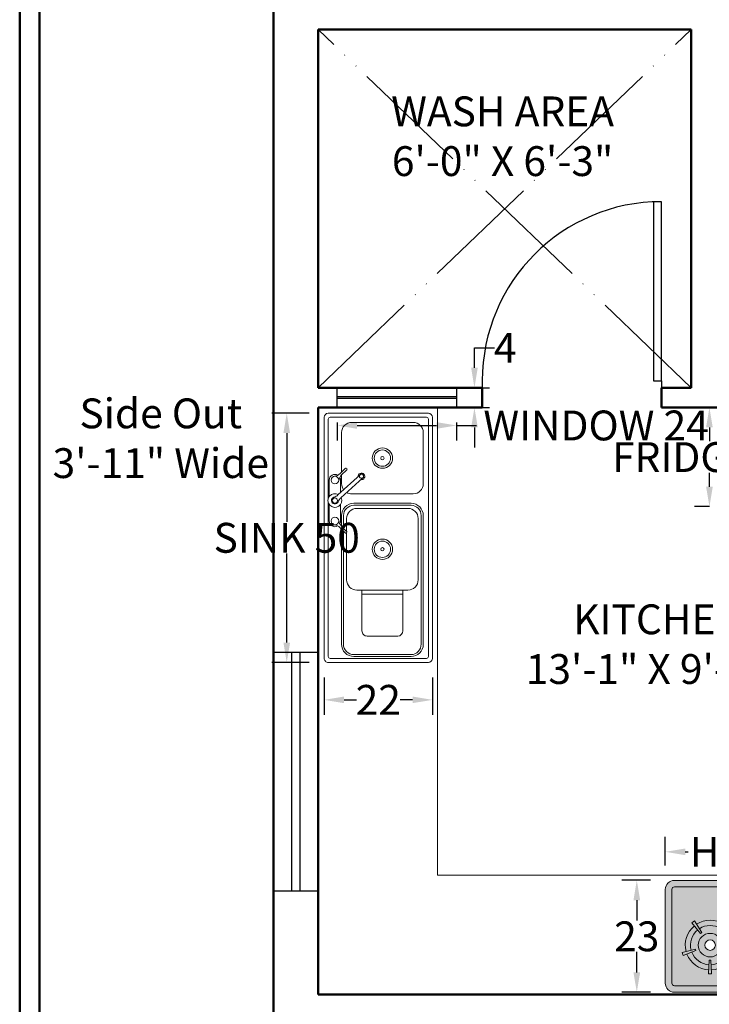
# Model space of a CAD drawing. Units: inches. Extents: x -466983 to 1020, y 324 to 318697.
# Tile 7 of 97: x 392 to 530, y 629 to 827. Entities that reach past the tile are written whole.
import ezdxf

# ---------------------------------------------------------------- set-up
doc = ezdxf.new("R2010")
doc.units = ezdxf.units.IN
doc.header["$MEASUREMENT"] = 0
doc.linetypes.add('ACAD_ISO05W100', pattern=[33, 24, -3, 0, -3, 0, -3])
for name, color, linetype, lineweight in [('A-ANNO-DIMS', 2, 'Continuous', 18), ('A-ANNO-SYMB', 252, 'ACAD_ISO05W100', 18), ('A-AREA-IDEN', 7, 'Continuous', 25), ('A-DOOR', 3, 'Continuous', 25), ('A-EQPM', 8, 'Continuous', 18), ('A-FLOR-FIXT', 9, 'Continuous', 18), ('A-FLOR-PATT', 252, 'Continuous', 13), ('A-GLAZ', 4, 'Continuous', 25), ('A-WALL', 7, 'Continuous', 50)]:
    doc.layers.add(name, color=color, linetype=linetype, lineweight=lineweight)
doc.styles.get("Standard").update_dxf_attribs({"font": 'arial.ttf'})
doc.dimstyles.get("Standard").update_dxf_attribs({"dimtxt": 6, "dimasz": 4, "dimexe": 3, "dimexo": 3, "dimgap": 0.09, "dimtad": 0, "dimtih": 1, "dimtoh": 1, "dimdec": 1, "dimzin": 0, "dimdsep": 46, "dimlunit": 3, "dimtxsty": 'Standard', "dimcen": 0.09, "dimadec": 0, "dimazin": 0, "dimtfac": 1, "dimtdec": 1, "dimtofl": 0, "dimtmove": 0, "dimatfit": 3, "dimfxl": 1, "dimtolj": 1, "dimtzin": 0, "dimarcsym": 0})

# ---------------------------------------------------------------- blocks, each defined once
blk = doc.blocks.new('Window 4 ft')
for p, q in [((1224.69, 893.77), (1233.69, 893.77)), ((1224.69, 845.77), (1224.69, 893.77)), ((1228.39, 845.77), (1228.39, 893.77)), ((1229.99, 893.77), (1229.99, 845.77)), ((1233.69, 893.77), (1233.69, 845.77)), ((1233.69, 845.77), (1224.69, 845.77))]:
    blk.add_line(p, q)
blk = doc.blocks.new('Window 4 inches')
for p, q in [((1548.16, 1036.06), (1572.16, 1036.06)), ((1548.16, 1032.06), (1548.16, 1036.06)), ((1572.16, 1036.06), (1572.16, 1032.06)), ((1548.16, 1034.26), (1572.16, 1034.26)), ((1572.16, 1033.86), (1548.16, 1033.86)), ((1572.16, 1032.06), (1548.16, 1032.06))]:
    blk.add_line(p, q)
blk = doc.blocks.new('*U39')
for p, q in [((0, 0), (0, -6)), ((-40, 0), (-40, -6))]:
    blk.add_line(p, q)
blk.add_lwpolyline([(0, 0), (0, 40), (-1.75, 40), (-1.75, 0)], close=True)
blk.add_arc((0, 0), 40, 90, 180)
blk = doc.blocks.new('Kitchen Sink')
at = {"color": 0}
for p, q in [((2657.86, 1007.76), (2657.86, 1030.74)), ((2714.14, 1031.68), (2658.8, 1031.68)), ((2713.67, 1030.74), (2659.27, 1030.74)), ((2715.08, 1007.76), (2715.08, 1030.74)), ((2658.8, 1030.27), (2658.8, 1008.23)), ((2674.04, 1029.57), (2662.32, 1029.57)), ((2710.89, 1029.57), (2681.35, 1029.57)), ((2710.89, 1029.1), (2681.35, 1029.1)), ((2696.12, 1028.39), (2682.05, 1028.39)), ((2714.14, 1008.23), (2714.14, 1030.27)), ((2659.97, 1027.22), (2659.97, 1013.15)), ((2676.39, 1027.22), (2676.39, 1013.15)), ((2678.54, 1026.75), (2678.54, 1013.62)), ((2679.01, 1026.75), (2679.01, 1013.62)), ((2679.71, 1026.05), (2679.71, 1014.32)), ((2698.47, 1026.05), (2698.47, 1014.32)), ((2713.28, 1013.62), (2713.28, 1026.75)), ((2713.71, 1013.62), (2713.71, 1026.75)), ((2698.47, 1024.88), (2707.85, 1024.88)), ((2699.4, 1024.88), (2699.4, 1015.5)), ((2709.02, 1016.67), (2709.02, 1023.7)), ((2676.63, 1009.99), (2672.02, 1015.05)), ((2677.32, 1010.63), (2672.71, 1015.68)), ((2698.47, 1015.5), (2707.85, 1015.5)), ((2671.4, 1010.81), (2662.32, 1010.81)), ((2671.7, 1010.5), (2670.59, 1011.62)), ((2672.03, 1010.83), (2670.93, 1011.95)), ((2674.04, 1010.81), (2672.05, 1010.81)), ((2673.22, 1010.59), (2676.08, 1010.59)), ((2678.79, 1010.59), (2682.6, 1010.59)), ((2681.35, 1011.24), (2684.25, 1011.24)), ((2681.35, 1010.81), (2683.82, 1010.81)), ((2684.99, 1011.98), (2682.05, 1011.98)), ((2683.81, 1010.81), (2684.94, 1011.91)), ((2684.14, 1010.47), (2685.27, 1011.58)), ((2684.49, 1010.81), (2710.89, 1010.81)), ((2684.92, 1011.24), (2710.89, 1011.24)), ((2696.12, 1011.98), (2685.33, 1011.98)), ((2673.22, 1007.97), (2677.03, 1007.97)), ((2678.79, 1007.97), (2682.6, 1007.97)), ((2658.8, 1006.82), (2714.14, 1006.82)), ((2659.27, 1007.76), (2677.51, 1007.76)), ((2678.32, 1007.76), (2713.67, 1007.76))]:
    blk.add_line(p, q, dxfattribs=at)
for centre, radius in [((2668.18, 1020.19), 2.34), ((2668.18, 1020.19), 1.88), ((2689.09, 1020.19), 2.34), ((2689.09, 1020.19), 1.88), ((2668.18, 1020.19), 0.399), ((2689.09, 1020.19), 0.399), ((2672.33, 1015.4), 0.471), ((2673.22, 1009.28), 0.878), ((2682.6, 1009.28), 0.878), ((2677.91, 1009.28), 0.601)]:
    blk.add_circle(centre, radius, dxfattribs=at)
for centre, radius, start, end in [((2658.8, 1030.74), 0.938, 90, 180), ((2659.27, 1030.27), 0.469, 90, 180), ((2713.67, 1030.27), 0.469, 0, 90), ((2714.14, 1030.74), 0.938, 0, 90), ((2662.32, 1027.22), 2.34, 90, 180), ((2674.04, 1027.22), 2.34, 0, 90), ((2681.35, 1026.75), 2.81, 90, 180), ((2681.35, 1026.75), 2.34, 90, 180), ((2682.05, 1026.05), 2.34, 90, 180), ((2696.12, 1026.05), 2.34, 0, 90), ((2710.89, 1026.75), 2.81, 0, 90), ((2710.87, 1026.68), 2.41, 1.6247, 89.3271), ((2707.85, 1023.7), 1.17, 0, 90), ((2672.37, 1015.37), 0.761, 350.3658, 274.3209), ((2707.85, 1016.67), 1.17, 270, 0), ((2662.32, 1013.15), 2.34, 180, 270), ((2674.04, 1013.15), 2.34, 330.2915, 0), ((2681.35, 1013.62), 2.81, 180, 270), ((2681.42, 1013.65), 2.41, 180.6729, 268.3753), ((2682.05, 1014.32), 2.34, 180, 270), ((2696.12, 1014.32), 2.34, 270, 0), ((2710.89, 1013.62), 2.81, 270, 0), ((2710.89, 1013.62), 2.38, 270, 0), ((2670.71, 1011.84), 0.248, 25.7239, 243.2674), ((2670.03, 1008.85), 2.34, 7.6523, 44.4956), ((2673.71, 1012.47), 2.34, 224.4956, 261.339), ((2673.22, 1009.28), 1.31, 90, 119.8816), ((2674.04, 1013.15), 2.34, 270, 307.0737), ((2677.91, 1009.28), 1.58, 149.6444, 115.0423), ((2679.06, 1012.21), 2.34, 222.3434, 248.6112), ((2682.17, 1012.48), 2.34, 277.6523, 314.4956), ((2682.6, 1009.28), 1.31, 59.1097, 90), ((2685.79, 1008.8), 2.34, 134.4956, 171.339), ((2685.16, 1011.8), 0.248, 295.7239, 153.2674), ((2696.12, 1014.32), 2.34, 270, 271.1456), ((2659.27, 1008.23), 0.469, 180, 270), ((2673.22, 1009.28), 1.31, 149.1097, 270), ((2674.9, 1008.41), 2.34, 16.0755, 42.3434), ((2677.91, 1009.28), 0.793, 196.0755, 68.6112), ((2682.6, 1009.28), 1.31, 270, 29.8816), ((2713.67, 1008.23), 0.469, 270, 0), ((2658.8, 1007.76), 0.938, 180, 270), ((2714.14, 1007.76), 0.938, 270, 0)]:
    blk.add_arc(centre, radius, start, end, dxfattribs=at)
blk = doc.blocks.new('Gas Stove')
h = blk.add_hatch(color=256)
h.dxf.hatch_style = 1
h.paths.add_polyline_path([(13032.81, 10915.17, 0.414214), (13029.34, 10918.64), (12963.86, 10918.64, 0.414214), (12960.39, 10915.17), (12960.39, 10879.45, 0.414214), (12963.86, 10875.98), (13029.34, 10875.98, 0.414214), (13032.81, 10879.45)])
h.paths.add_polyline_path([(13030.33, 10879.45, -0.414214), (13029.34, 10878.46), (12963.86, 10878.46, -0.414214), (12962.87, 10879.45), (12962.87, 10915.17, -0.414214), (12963.86, 10916.16), (13029.34, 10916.16, -0.414214), (13030.33, 10915.17)], flags=16)
h.paths.add_polyline_path([(13026, 10904.63), (13026.36, 10903.5), (13024.89, 10903.11, -0.295473), (13021.71, 10893.34), (13022.68, 10892.15), (13021.71, 10891.45), (13020.89, 10892.74, -0.295473), (13010.61, 10892.74), (13009.78, 10891.45), (13008.82, 10892.15), (13009.79, 10893.34, -0.295473), (13006.61, 10903.11), (13005.13, 10903.5), (13005.5, 10904.63), (13006.93, 10904.08, -0.295473), (13015.24, 10910.12), (13015.15, 10911.64), (13016.34, 10911.64), (13016.26, 10910.12, -0.295473), (13024.57, 10904.08)], flags=0)
h.paths.add_polyline_path([(13020.24, 10900.68, -1), (13011.25, 10900.68, -1)], flags=0)
h.paths.add_polyline_path([(13017.76, 10900.68, -1), (13013.73, 10900.68, -1)], flags=0)
h.paths.add_polyline_path([(13001.07, 10889.32), (13001.07, 10886.1), (12992.13, 10886.1), (12992.13, 10889.32)], flags=0)
h.paths.add_polyline_path([(13001.08, 10880.42), (13001.08, 10880.13), (13000.33, 10880.13), (13000.33, 10880.42, -0.820702), (13000.33, 10884.1), (13000.33, 10884.41), (13001.08, 10884.41), (13001.08, 10884.1, -0.816133)], flags=0)
h.paths.add_polyline_path([(12988.06, 10903.5), (12986.59, 10903.11, -0.295473), (12983.41, 10893.34), (12984.38, 10892.15), (12983.41, 10891.45), (12982.59, 10892.74, -0.295473), (12972.31, 10892.74), (12971.48, 10891.45), (12970.52, 10892.15), (12971.49, 10893.34, -0.295473), (12968.31, 10903.11), (12966.83, 10903.5), (12967.2, 10904.63), (12968.63, 10904.08, -0.295473), (12976.94, 10910.12), (12976.85, 10911.64), (12978.04, 10911.64), (12977.96, 10910.12, -0.295473), (12986.27, 10904.08), (12987.7, 10904.63)], flags=0)
h.paths.add_polyline_path([(12992.89, 10880.42), (12992.89, 10880.13), (12992.14, 10880.13), (12992.14, 10880.42, -0.816133), (12992.14, 10884.1), (12992.14, 10884.41), (12992.89, 10884.41), (12992.89, 10884.1, -0.820702)], flags=0)
h.paths.add_polyline_path([(12981.94, 10900.68, -1), (12972.95, 10900.68, -1)], flags=0)
h.paths.add_polyline_path([(12979.46, 10900.68, -1), (12975.43, 10900.68, -1)], flags=0)
h = blk.add_hatch(color=0)
h.dxf.hatch_style = 1
h.set_gradient(color1=(192, 192, 192), color2=(0, 0, 0))
h.paths.add_polyline_path([(13030.33, 10915.17, 0.414214), (13029.34, 10916.16), (12963.86, 10916.16, 0.414214), (12962.87, 10915.17), (12962.87, 10879.45, 0.414214), (12963.86, 10878.46), (13029.34, 10878.46, 0.414214), (13030.33, 10879.45)])
h.paths.add_polyline_path([(12987.7, 10904.63), (12988.06, 10903.5), (12986.59, 10903.11, -0.295473), (12983.41, 10893.34), (12984.38, 10892.15), (12983.41, 10891.45), (12982.59, 10892.74, -0.295473), (12972.31, 10892.74), (12971.48, 10891.45), (12970.52, 10892.15), (12971.49, 10893.34, -0.295473), (12968.31, 10903.11), (12966.83, 10903.5), (12967.2, 10904.63), (12968.63, 10904.08, -0.295473), (12976.94, 10910.12), (12976.85, 10911.64), (12978.04, 10911.64), (12977.96, 10910.12, -0.295473), (12986.27, 10904.08)], flags=16)
h.paths.add_polyline_path([(13005.5, 10904.63), (13006.93, 10904.08, -0.295473), (13015.24, 10910.12), (13015.15, 10911.64), (13016.34, 10911.64), (13016.26, 10910.12, -0.295473), (13024.57, 10904.08), (13026, 10904.63), (13026.36, 10903.5), (13024.89, 10903.11, -0.295473), (13021.71, 10893.34), (13022.68, 10892.15), (13021.71, 10891.45), (13020.89, 10892.74, -0.295473), (13010.61, 10892.74), (13009.78, 10891.45), (13008.82, 10892.15), (13009.79, 10893.34, -0.295473), (13006.61, 10903.11), (13005.13, 10903.5)], flags=16)
h.paths.add_polyline_path([(12981.94, 10900.68, -1), (12972.95, 10900.68, -1)], flags=0)
h.paths.add_polyline_path([(12979.46, 10900.68, -1), (12975.43, 10900.68, -1)], flags=0)
h.paths.add_polyline_path([(13020.24, 10900.68, -1), (13011.25, 10900.68, -1)], flags=0)
h.paths.add_polyline_path([(13017.76, 10900.68, -1), (13013.73, 10900.68, -1)], flags=0)
h.paths.add_polyline_path([(13001.07, 10889.32), (13001.07, 10886.1), (12992.13, 10886.1), (12992.13, 10889.32)], flags=16)
h.paths.add_polyline_path([(12992.89, 10884.41), (12992.89, 10884.1, -0.820702), (12992.89, 10880.42), (12992.89, 10880.13), (12992.14, 10880.13), (12992.14, 10880.42, -0.816133), (12992.14, 10884.1), (12992.14, 10884.41)], flags=16)
h.paths.add_polyline_path([(13000.33, 10884.41), (13001.08, 10884.41), (13001.08, 10884.1, -0.816133), (13001.08, 10880.42), (13001.08, 10880.13), (13000.33, 10880.13), (13000.33, 10880.42, -0.820702), (13000.33, 10884.1)], flags=16)
h.paths.add_polyline_path([(13022.97, 10902.61), (13021.31, 10902.17), (13021.12, 10902.73), (13022.72, 10903.36, 0.295997), (13016.14, 10908.14), (13016.04, 10906.42), (13015.45, 10906.42), (13015.35, 10908.14, 0.295997), (13008.78, 10903.36), (13010.38, 10902.73), (13010.19, 10902.17), (13008.53, 10902.61, 0.295997), (13011.04, 10894.87), (13012.13, 10896.2), (13012.61, 10895.85), (13011.68, 10894.41, 0.295997), (13019.82, 10894.41), (13018.89, 10895.85), (13019.37, 10896.2), (13020.45, 10894.87, 0.295997)], flags=0)
h = blk.add_hatch(color=256)
h.dxf.hatch_style = 1
h.set_gradient(color1=(237, 238, 153), color2=(128, 128, 128), name='INVSPHERICAL')
h.paths.add_polyline_path([(13030.33, 10915.17, 0.414214), (13029.34, 10916.16), (12963.86, 10916.16, 0.414214), (12962.87, 10915.17), (12962.87, 10879.45, 0.414214), (12963.86, 10878.46), (13029.34, 10878.46, 0.414214), (13030.33, 10879.45)])
h.paths.add_polyline_path([(12986.27, 10904.08), (12987.7, 10904.63), (12988.06, 10903.5), (12986.59, 10903.11, -0.295473), (12983.41, 10893.34), (12984.38, 10892.15), (12983.41, 10891.45), (12982.59, 10892.74, -0.295473), (12972.31, 10892.74), (12971.48, 10891.45), (12970.52, 10892.15), (12971.49, 10893.34, -0.295473), (12968.31, 10903.11), (12966.83, 10903.5), (12967.2, 10904.63), (12968.63, 10904.08, -0.295473), (12976.94, 10910.12), (12976.85, 10911.64), (12978.04, 10911.64), (12977.96, 10910.12, -0.295473)], flags=16)
h.paths.add_polyline_path([(12981.94, 10900.68, -1), (12972.95, 10900.68, -1)], flags=0)
h.paths.add_polyline_path([(12979.46, 10900.68, -1), (12975.43, 10900.68, -1)], flags=0)
h.paths.add_polyline_path([(13005.5, 10904.63), (13006.93, 10904.08, -0.295473), (13015.24, 10910.12), (13015.15, 10911.64), (13016.34, 10911.64), (13016.26, 10910.12, -0.295473), (13024.57, 10904.08), (13026, 10904.63), (13026.36, 10903.5), (13024.89, 10903.11, -0.295473), (13021.71, 10893.34), (13022.68, 10892.15), (13021.71, 10891.45), (13020.89, 10892.74, -0.295473), (13010.61, 10892.74), (13009.78, 10891.45), (13008.82, 10892.15), (13009.79, 10893.34, -0.295473), (13006.61, 10903.11), (13005.13, 10903.5)], flags=16)
h.paths.add_polyline_path([(12992.13, 10889.32), (13001.07, 10889.32), (13001.07, 10886.1), (12992.13, 10886.1)], flags=16)
h.paths.add_polyline_path([(13020.24, 10900.68, -1), (13011.25, 10900.68, -1)], flags=0)
h.paths.add_polyline_path([(13017.76, 10900.68, -1), (13013.73, 10900.68, -1)], flags=0)
h.paths.add_polyline_path([(12992.14, 10884.41), (12992.89, 10884.41), (12992.89, 10884.1, -0.820702), (12992.89, 10880.42), (12992.89, 10880.13), (12992.14, 10880.13), (12992.14, 10880.42, -0.816133), (12992.14, 10884.1)], flags=16)
h.paths.add_polyline_path([(13000.33, 10884.41), (13001.08, 10884.41), (13001.08, 10884.1, -0.816133), (13001.08, 10880.42), (13001.08, 10880.13), (13000.33, 10880.13), (13000.33, 10880.42, -0.820702), (13000.33, 10884.1)], flags=16)
h = blk.add_hatch(color=256)
h.dxf.hatch_style = 1
h.paths.add_polyline_path([(13005.5, 10904.63), (13005.13, 10903.5), (13010.19, 10902.17), (13010.38, 10902.73)])
h.paths.add_polyline_path([(13012.61, 10895.85), (13012.13, 10896.2), (13008.82, 10892.15), (13009.78, 10891.45)])
h.paths.add_polyline_path([(13019.37, 10896.2), (13018.89, 10895.85), (13021.71, 10891.45), (13022.68, 10892.15)])
h.paths.add_polyline_path([(13026.36, 10903.5), (13026, 10904.63), (13021.12, 10902.73), (13021.31, 10902.17)])
h.paths.add_polyline_path([(13016.34, 10911.64), (13015.15, 10911.64), (13015.45, 10906.42), (13016.04, 10906.42)])
h.paths.add_polyline_path([(12988.06, 10903.5), (12987.7, 10904.63), (12982.82, 10902.73), (12983.01, 10902.17)])
h.paths.add_polyline_path([(12978.04, 10911.64), (12976.85, 10911.64), (12977.15, 10906.42), (12977.74, 10906.42)])
h.paths.add_polyline_path([(12981.07, 10896.2), (12980.59, 10895.85), (12983.41, 10891.45), (12984.38, 10892.15)])
h.paths.add_polyline_path([(12974.31, 10895.85), (12973.83, 10896.2), (12970.52, 10892.15), (12971.48, 10891.45)])
h.paths.add_polyline_path([(12967.2, 10904.63), (12966.83, 10903.5), (12971.89, 10902.17), (12972.08, 10902.73)])
h = blk.add_hatch(color=256)
h.dxf.hatch_style = 1
h.paths.add_polyline_path([(12986.59, 10903.11), (12984.67, 10902.61, -0.295997), (12982.15, 10894.87), (12983.41, 10893.34, 0.295473)])
h.paths.add_polyline_path([(12977.96, 10910.12), (12977.84, 10908.14, -0.295997), (12984.42, 10903.36), (12986.27, 10904.08, 0.295473)])
h.paths.add_polyline_path([(12977.06, 10908.14), (12976.94, 10910.12, 0.295473), (12968.63, 10904.08), (12970.48, 10903.36, -0.295997)])
h.paths.add_polyline_path([(12970.23, 10902.61), (12968.31, 10903.11, 0.295473), (12971.49, 10893.34), (12972.75, 10894.87, -0.295997)])
h.paths.add_polyline_path([(12982.59, 10892.74), (12981.52, 10894.41, -0.295997), (12973.38, 10894.41), (12972.31, 10892.74, 0.295473)])
h.paths.add_polyline_path([(13016.26, 10910.12), (13016.14, 10908.14, -0.295997), (13022.72, 10903.36), (13024.57, 10904.08, 0.295473)])
h.paths.add_polyline_path([(13024.89, 10903.11), (13022.97, 10902.61, -0.295997), (13020.45, 10894.87), (13021.71, 10893.34, 0.295473)])
h.paths.add_polyline_path([(13020.89, 10892.74), (13019.82, 10894.41, -0.295997), (13011.68, 10894.41), (13010.61, 10892.74, 0.295473)])
h.paths.add_polyline_path([(13008.53, 10902.61), (13006.61, 10903.11, 0.295473), (13009.79, 10893.34), (13011.04, 10894.87, -0.295997)])
h.paths.add_polyline_path([(13015.35, 10908.14), (13015.24, 10910.12, 0.295473), (13006.93, 10904.08), (13008.78, 10903.36, -0.295997)])
h = blk.add_hatch(color=0)
h.dxf.hatch_style = 1
h.set_gradient(color1=(192, 192, 192), color2=(0, 0, 0), name='CYLINDER')
h.paths.add_polyline_path([(13022.97, 10902.61), (13021.31, 10902.17), (13021.12, 10902.73), (13022.72, 10903.36, 0.295997), (13016.14, 10908.14), (13016.04, 10906.42), (13015.45, 10906.42), (13015.35, 10908.14, 0.295997), (13008.78, 10903.36), (13010.38, 10902.73), (13010.19, 10902.17), (13008.53, 10902.61, 0.295997), (13011.04, 10894.87), (13012.13, 10896.2), (13012.61, 10895.85), (13011.68, 10894.41, 0.295997), (13019.82, 10894.41), (13018.89, 10895.85), (13019.37, 10896.2), (13020.45, 10894.87, 0.295997)])
h.paths.add_polyline_path([(13011.25, 10900.68, -1), (13020.24, 10900.68, -1)], flags=16)
h.paths.add_polyline_path([(13013.73, 10900.68, -1), (13017.76, 10900.68, -1)], flags=0)
h.paths.add_polyline_path([(12984.67, 10902.61), (12983.01, 10902.17), (12982.82, 10902.73), (12984.42, 10903.36, 0.295997), (12977.84, 10908.14), (12977.74, 10906.42), (12977.15, 10906.42), (12977.06, 10908.14, 0.295997), (12970.48, 10903.36), (12972.08, 10902.73), (12971.89, 10902.17), (12970.23, 10902.61, 0.295997), (12972.75, 10894.87), (12973.83, 10896.2), (12974.31, 10895.85), (12973.38, 10894.41, 0.295997), (12981.52, 10894.41), (12980.59, 10895.85), (12981.07, 10896.2), (12982.15, 10894.87, 0.295997)])
h.paths.add_polyline_path([(12972.95, 10900.68, -1), (12981.94, 10900.68, -1)], flags=16)
h.paths.add_polyline_path([(12975.43, 10900.68, -1), (12979.46, 10900.68, -1)], flags=0)
h = blk.add_hatch(color=0)
h.dxf.hatch_style = 1
h.set_gradient(color1=(0, 0, 255), color2=(255, 0, 0), name='CYLINDER')
h.paths.add_polyline_path([(13011.25, 10900.68, 1), (13020.24, 10900.68, 1)])
h.paths.add_polyline_path([(13017.76, 10900.68, -1), (13013.73, 10900.68, -1)], flags=16)
h.paths.add_polyline_path([(12972.95, 10900.68, 1), (12981.94, 10900.68, 1)])
h.paths.add_polyline_path([(12979.46, 10900.68, -1), (12975.43, 10900.68, -1)], flags=16)
h = blk.add_hatch(color=256)
h.dxf.hatch_style = 1
h.paths.add_polyline_path([(13001.07, 10889.32), (12992.13, 10889.32), (12992.13, 10886.1), (13001.07, 10886.1)])
h.paths.add_polyline_path([(13001.08, 10884.41), (13000.33, 10884.41), (13000.33, 10880.13), (13001.08, 10880.13)])
h.paths.add_polyline_path([(12992.89, 10884.41), (12992.14, 10884.41), (12992.14, 10880.13), (12992.89, 10880.13)])
h = blk.add_hatch(color=0)
h.dxf.hatch_style = 1
h.set_gradient(color1=(0, 0, 255), color2=(255, 0, 0), name='CYLINDER')
h.paths.add_polyline_path([(13001.08, 10884.1), (13001.08, 10880.42, 0.816133)])
h.paths.add_polyline_path([(13000.33, 10884.1, 0.820702), (13000.33, 10880.42)])
h.paths.add_polyline_path([(12992.89, 10884.1), (12992.89, 10880.42, 0.820702)])
h.paths.add_polyline_path([(12992.14, 10884.1, 0.816133), (12992.14, 10880.42)])
at = {"color": 0}
for p, q in [((12963.86, 10918.64), (13029.34, 10918.64)), ((12960.39, 10879.45), (12960.39, 10915.17)), ((12962.87, 10879.45), (12962.87, 10915.17)), ((12963.86, 10916.16), (13029.34, 10916.16)), ((13030.33, 10915.17), (13030.33, 10879.45)), ((13032.81, 10915.17), (13032.81, 10879.45)), ((12976.85, 10911.64), (12977.15, 10906.42)), ((12976.85, 10911.64), (12978.04, 10911.64)), ((12978.04, 10911.64), (12977.74, 10906.42)), ((13015.15, 10911.64), (13015.45, 10906.42)), ((13016.34, 10911.64), (13015.15, 10911.64)), ((13016.34, 10911.64), (13016.04, 10906.42)), ((12977.15, 10906.42), (12977.74, 10906.42)), ((13016.04, 10906.42), (13015.45, 10906.42)), ((12966.83, 10903.5), (12967.2, 10904.63)), ((12966.83, 10903.5), (12971.89, 10902.17)), ((12967.2, 10904.63), (12972.08, 10902.73)), ((12971.89, 10902.17), (12972.08, 10902.73)), ((12987.7, 10904.63), (12982.82, 10902.73)), ((12982.82, 10902.73), (12983.01, 10902.17)), ((12988.06, 10903.5), (12983.01, 10902.17)), ((12987.7, 10904.63), (12988.06, 10903.5)), ((13005.5, 10904.63), (13005.13, 10903.5)), ((13005.13, 10903.5), (13010.19, 10902.17)), ((13005.5, 10904.63), (13010.38, 10902.73)), ((13010.38, 10902.73), (13010.19, 10902.17)), ((13026, 10904.63), (13021.12, 10902.73)), ((13021.31, 10902.17), (13021.12, 10902.73)), ((13026.36, 10903.5), (13021.31, 10902.17)), ((13026.36, 10903.5), (13026, 10904.63)), ((12970.52, 10892.15), (12973.83, 10896.2)), ((12971.48, 10891.45), (12974.31, 10895.85)), ((12974.31, 10895.85), (12973.83, 10896.2)), ((12981.07, 10896.2), (12980.59, 10895.85)), ((12983.41, 10891.45), (12980.59, 10895.85)), ((12984.38, 10892.15), (12981.07, 10896.2)), ((13008.82, 10892.15), (13012.13, 10896.2)), ((13009.78, 10891.45), (13012.61, 10895.85)), ((13012.13, 10896.2), (13012.61, 10895.85)), ((13018.89, 10895.85), (13019.37, 10896.2)), ((13021.71, 10891.45), (13018.89, 10895.85)), ((13022.68, 10892.15), (13019.37, 10896.2)), ((12971.48, 10891.45), (12970.52, 10892.15)), ((12984.38, 10892.15), (12983.41, 10891.45)), ((13008.82, 10892.15), (13009.78, 10891.45)), ((13021.71, 10891.45), (13022.68, 10892.15)), ((12992.13, 10889.32), (12992.13, 10886.1)), ((13001.07, 10889.32), (12992.13, 10889.32)), ((13001.07, 10886.1), (13001.07, 10889.32)), ((12992.13, 10886.1), (13001.07, 10886.1)), ((12992.14, 10884.41), (12992.14, 10880.13)), ((12992.89, 10884.41), (12992.14, 10884.41)), ((12992.89, 10880.13), (12992.89, 10884.41)), ((13000.33, 10884.41), (13001.08, 10884.41)), ((13000.33, 10880.13), (13000.33, 10884.41)), ((13001.08, 10884.41), (13001.08, 10880.13)), ((12992.14, 10880.13), (12992.89, 10880.13)), ((13001.08, 10880.13), (13000.33, 10880.13)), ((13029.34, 10878.46), (12963.86, 10878.46)), ((13029.34, 10875.98), (12963.86, 10875.98))]:
    blk.add_line(p, q, dxfattribs=at)
for centre, radius in [((12977.45, 10900.68), 4.49), ((12977.45, 10900.68), 2.01), ((13015.75, 10900.68), 4.49), ((13015.75, 10900.68), 2.01)]:
    blk.add_circle(centre, radius, dxfattribs=at)
for centre, radius, start, end in [((12963.86, 10915.17), 3.47, 90, 180), ((13029.34, 10915.17), 3.47, 0, 90), ((12963.86, 10915.17), 0.992, 90, 180), ((13029.34, 10915.17), 0.992, 0, 90), ((12977.45, 10900.68), 9.46, 93.078, 158.922), ((12977.45, 10900.68), 9.46, 21.078, 86.922), ((13015.75, 10900.68), 9.46, 93.078, 158.922), ((13015.75, 10900.68), 9.46, 21.078, 86.922), ((12977.45, 10900.68), 7.47, 93.0228, 158.9772), ((12977.45, 10900.68), 7.47, 21.0228, 86.9772), ((13015.75, 10900.68), 7.47, 93.0228, 158.9772), ((13015.75, 10900.68), 7.47, 21.0228, 86.9772), ((12977.45, 10900.68), 9.46, 165.078, 230.922), ((12977.45, 10900.68), 7.47, 165.0228, 230.9772), ((12977.45, 10900.68), 7.47, 309.0228, 14.9772), ((12977.45, 10900.68), 9.46, 309.078, 14.922), ((13015.75, 10900.68), 9.46, 165.078, 230.922), ((13015.75, 10900.68), 7.47, 165.0228, 230.9772), ((13015.75, 10900.68), 7.47, 309.0228, 14.9772), ((13015.75, 10900.68), 9.46, 309.078, 14.922), ((12977.45, 10900.68), 9.46, 237.078, 302.922), ((12977.45, 10900.68), 7.47, 237.0228, 302.9772), ((13015.75, 10900.68), 9.46, 237.078, 302.922), ((13015.75, 10900.68), 7.47, 237.0228, 302.9772), ((12992.52, 10882.26), 1.88, 101.5619, 258.4381), ((12992.52, 10882.26), 1.88, 281.2484, 78.7516), ((13000.7, 10882.26), 1.88, 101.2484, 258.7516), ((13000.7, 10882.26), 1.88, 281.5619, 78.4381), ((12963.86, 10879.45), 3.47, 180, 270), ((12963.86, 10879.45), 0.992, 180, 270), ((13029.34, 10879.45), 0.992, 270, 0), ((13029.34, 10879.45), 3.47, 270, 0)]:
    blk.add_arc(centre, radius, start, end, dxfattribs=at)
blk = doc.blocks.new('*D67')
at = {"layer": 'A-ANNO-DIMS', "color": 0, "lineweight": -2, "transparency": 16777216}
for p, q in [((455.63, 745.94), (455.63, 742.34)), ((459.63, 745.34), (475.63, 745.34)), ((479.63, 745.94), (479.63, 742.34)), ((479.63, 745.34), (483.63, 745.34))]:
    blk.add_line(p, q, dxfattribs=at)
at = {"layer": 'A-ANNO-DIMS', "color": 0, "transparency": 16777216}
for points in [[(459.63, 746), (459.63, 744.67), (455.63, 745.34)], [(475.63, 746), (475.63, 744.67), (479.63, 745.34)]]:
    blk.add_solid(points, dxfattribs=at)
at = {"layer": 'Defpoints', "color": 0, "transparency": 16777216}
for p in [(455.63, 748.94), (479.63, 748.94), (479.63, 745.34)]:
    blk.add_point(p, dxfattribs=at)
at = {"layer": 'A-ANNO-DIMS', "color": 0, "transparency": 16777216, "insert": (507.68, 745.34), "char_height": 6, "attachment_point": 5}
blk.add_mtext('\\A1;WINDOW 24', dxfattribs=at)
blk = doc.blocks.new('*D68')
at = {"layer": 'A-ANNO-DIMS', "color": 0, "lineweight": -2, "transparency": 16777216}
for p, q in [((483.23, 756.94), (483.23, 760.94)), ((483.23, 760.94), (487.23, 760.94)), ((482.63, 752.94), (486.23, 752.94)), ((482.63, 748.94), (486.23, 748.94)), ((483.23, 744.94), (483.23, 740.94))]:
    blk.add_line(p, q, dxfattribs=at)
at = {"layer": 'A-ANNO-DIMS', "color": 0, "transparency": 16777216}
for points in [[(482.56, 756.94), (483.9, 756.94), (483.23, 752.94)], [(482.56, 744.94), (483.9, 744.94), (483.23, 748.94)]]:
    blk.add_solid(points, dxfattribs=at)
at = {"layer": 'Defpoints', "color": 0, "transparency": 16777216}
for p in [(479.63, 752.94), (483.23, 752.94), (479.63, 748.94)]:
    blk.add_point(p, dxfattribs=at)
at = {"layer": 'A-ANNO-DIMS', "color": 0, "transparency": 16777216, "insert": (489.4, 760.94), "char_height": 6, "attachment_point": 5}
blk.add_mtext('\\A1;4', dxfattribs=at)
blk = doc.blocks.new('*D105')
at = {"layer": 'A-ANNO-DIMS', "color": 0, "lineweight": -2, "transparency": 16777216}
for p, q in [((450.01, 747.81), (442.49, 747.81)), ((445.49, 743.81), (445.49, 725.94)), ((445.49, 701.68), (445.49, 719.56)), ((450.01, 697.68), (442.49, 697.68))]:
    blk.add_line(p, q, dxfattribs=at)
at = {"layer": 'A-ANNO-DIMS', "color": 0, "transparency": 16777216}
for points in [[(444.83, 743.81), (446.16, 743.81), (445.49, 747.81)], [(444.83, 701.68), (446.16, 701.68), (445.49, 697.68)]]:
    blk.add_solid(points, dxfattribs=at)
at = {"layer": 'Defpoints', "color": 0, "transparency": 16777216}
for p in [(453.01, 747.81), (445.49, 697.68), (453.01, 697.68)]:
    blk.add_point(p, dxfattribs=at)
at = {"layer": 'A-ANNO-DIMS', "color": 0, "transparency": 16777216, "insert": (445.49, 722.75), "char_height": 6, "attachment_point": 5}
blk.add_mtext('\\A1;SINK 50', dxfattribs=at)
blk = doc.blocks.new('*D106')
at = {"layer": 'A-ANNO-DIMS', "color": 0, "lineweight": -2, "transparency": 16777216}
for p, q in [((453.01, 694.68), (453.01, 687.16)), ((474.79, 694.68), (474.79, 687.16)), ((457.01, 690.16), (459.49, 690.16)), ((470.79, 690.16), (468.31, 690.16))]:
    blk.add_line(p, q, dxfattribs=at)
at = {"layer": 'A-ANNO-DIMS', "color": 0, "transparency": 16777216}
for points in [[(457.01, 690.83), (457.01, 689.5), (453.01, 690.16)], [(470.79, 690.83), (470.79, 689.5), (474.79, 690.16)]]:
    blk.add_solid(points, dxfattribs=at)
at = {"layer": 'Defpoints', "color": 0, "transparency": 16777216}
for p in [(453.01, 697.68), (474.79, 697.68), (474.79, 690.16)]:
    blk.add_point(p, dxfattribs=at)
at = {"layer": 'A-ANNO-DIMS', "color": 0, "transparency": 16777216, "insert": (463.9, 690.16), "char_height": 6, "attachment_point": 5}
blk.add_mtext('\\A1;22', dxfattribs=at)
blk = doc.blocks.new('*D107')
at = {"layer": 'A-ANNO-DIMS', "color": 0, "lineweight": -2, "transparency": 16777216}
for p, q in [((521.6, 656.87), (521.6, 662.6)), ((559.81, 656.87), (559.81, 662.6)), ((525.6, 659.6), (526.23, 659.6)), ((555.81, 659.6), (555.18, 659.6))]:
    blk.add_line(p, q, dxfattribs=at)
at = {"layer": 'A-ANNO-DIMS', "color": 0, "transparency": 16777216}
for points in [[(525.6, 660.27), (525.6, 658.93), (521.6, 659.6)], [(555.81, 660.27), (555.81, 658.93), (559.81, 659.6)]]:
    blk.add_solid(points, dxfattribs=at)
at = {"layer": 'Defpoints', "color": 0, "transparency": 16777216}
for p in [(521.6, 659.6), (521.6, 653.87), (559.81, 653.87)]:
    blk.add_point(p, dxfattribs=at)
at = {"layer": 'A-ANNO-DIMS', "color": 0, "transparency": 16777216, "insert": (540.71, 659.6), "char_height": 6, "attachment_point": 5}
blk.add_mtext('\\A1;HOB 38', dxfattribs=at)
blk = doc.blocks.new('*D108')
at = {"layer": 'A-ANNO-DIMS', "color": 0, "lineweight": -2, "transparency": 16777216}
for p, q in [((518.6, 653.87), (512.87, 653.87)), ((515.87, 649.87), (515.87, 645.77)), ((515.87, 635.36), (515.87, 639.46)), ((518.6, 631.36), (512.87, 631.36))]:
    blk.add_line(p, q, dxfattribs=at)
at = {"layer": 'A-ANNO-DIMS', "color": 0, "transparency": 16777216}
for points in [[(515.2, 649.87), (516.54, 649.87), (515.87, 653.87)], [(515.2, 635.36), (516.54, 635.36), (515.87, 631.36)]]:
    blk.add_solid(points, dxfattribs=at)
at = {"layer": 'Defpoints', "color": 0, "transparency": 16777216}
for p in [(521.6, 653.87), (515.87, 631.36), (521.6, 631.36)]:
    blk.add_point(p, dxfattribs=at)
at = {"layer": 'A-ANNO-DIMS', "color": 0, "transparency": 16777216, "insert": (515.87, 642.61), "char_height": 6, "attachment_point": 5}
blk.add_mtext('\\A1;23', dxfattribs=at)
blk = doc.blocks.new('*D109')
at = {"layer": 'A-ANNO-DIMS', "color": 0, "lineweight": -2, "transparency": 16777216}
for p, q in [((530.46, 748.94), (527.47, 748.94)), ((530.47, 744.94), (530.47, 742.17)), ((530.47, 733.02), (530.47, 735.79)), ((530.46, 729.02), (527.47, 729.02))]:
    blk.add_line(p, q, dxfattribs=at)
at = {"layer": 'A-ANNO-DIMS', "color": 0, "transparency": 16777216}
for points in [[(529.8, 744.94), (531.14, 744.94), (530.47, 748.94)], [(529.8, 733.02), (531.14, 733.02), (530.47, 729.02)]]:
    blk.add_solid(points, dxfattribs=at)
at = {"layer": 'Defpoints', "color": 0, "transparency": 16777216}
for p in [(533.46, 748.94), (530.47, 729.02), (533.46, 729.02)]:
    blk.add_point(p, dxfattribs=at)
at = {"layer": 'A-ANNO-DIMS', "color": 0, "transparency": 16777216, "insert": (530.47, 738.98), "char_height": 6, "attachment_point": 5}
blk.add_mtext('\\A1;FRIDGE 20', dxfattribs=at)

msp = doc.modelspace()

# ---------------------------------------------------------------- hatches: boundary and pattern name
at = {"layer": 'A-FLOR-PATT', "transparency": 33554572}
h = msp.add_hatch(dxfattribs=at)
h.set_pattern_fill('ANSI37', color=256, scale=30)
h.set_pattern_definition([(45, (-1212.4137, -290.035), (-2.6516504, 2.6516504), []), (135, (-1212.4137, -290.035), (-2.6516504, -2.6516504), [])])
h.paths.add_polyline_path([(901.81, 1075.94), (900.61, 1075.94), (900.61, 1065.39), (899.39, 1065.39), (898.09, 1065.39), (892.84, 1058.71, -0.258377), (892.19, 1058.35), (879.98, 1058.35, -0.20177), (879.44, 1058.58), (874.08, 1065.39), (872.78, 1065.39), (871.56, 1065.39), (871.56, 1075.94), (813.81, 1075.94), (813.81, 1044.79), (832.39, 1044.79, -0.394795), (848.66, 1028.54), (848.66, 1009.94), (901.81, 1009.94), (901.81, 1015.94), (901.31, 1015.94), (871.31, 1015.94), (871.31, 1017.25), (871.33, 1017.25, -0.401453), (901.31, 1045.94), (901.81, 1045.94)])
edge = h.paths.add_edge_path(flags=16)
edge.add_line((847.77, 1068.95), (847.77, 1073.71))
edge.add_arc((849.23, 1073.71), 1.45, 90, 180, ccw=False)
edge.add_line((849.23, 1075.16), (864.49, 1075.16))
edge.add_arc((864.49, 1073.71), 1.45, 0, 90, ccw=False)
edge.add_line((865.95, 1073.71), (865.95, 1069))
edge.add_arc((832.64, 1068.98), 33.3, -20.6123, 0.0472, ccw=False)
edge.add_ellipse((856.86, 1058.48), major_axis=(0, 10.21), ratio=0.685919, start_angle=100.0088, end_angle=259.9912, ccw=False)
edge.add_arc((881.07, 1068.98), 33.3, 180.0472, 200.6123, ccw=False)
h.paths.add_polyline_path([(853.15, 1066.48), (853.15, 1066.45), (853.15, 1066.45, 0.433107), (852.92, 1066.68), (852.92, 1066.45), (853.15, 1066.45), (853.15, 1066.48), (853.09, 1066.61, 0.697939), (852.7, 1066.45), (852.7, 1066.45), (852.7, 1066.48), (852.92, 1067), (852.92, 1066.68, -0.396254)], flags=0)
h.paths.add_polyline_path([(861.02, 1066.48), (861.02, 1066.45), (861.02, 1066.45, 0.416404), (860.8, 1066.68), (860.8, 1066.45), (861.02, 1066.45), (861.02, 1066.48), (860.97, 1066.61, 0.713344), (860.57, 1066.45), (860.57, 1066.45), (860.57, 1066.48), (860.8, 1067), (860.8, 1066.68, -0.379973)], flags=0)
edge = h.paths.add_edge_path(flags=0)
edge.add_spline(control_points=[(861.13, 1065.79), (861.47, 1065.25), (861.61, 1065.02), (861.98, 1064.37), (862.19, 1063.94), (862.56, 1063.04), (862.72, 1062.56), (862.99, 1061.58), (863.09, 1061.07), (863.25, 1060.03), (863.29, 1059.5), (863.33, 1058.44), (863.32, 1057.91), (863.24, 1056.85), (863.17, 1056.33), (862.97, 1055.31), (862.84, 1054.81), (862.54, 1053.85), (862.36, 1053.39), (861.95, 1052.52), (861.73, 1052.12), (861.23, 1051.36), (860.97, 1051.02), (860.4, 1050.39), (860.11, 1050.12), (859.49, 1049.65), (859.18, 1049.45), (858.53, 1049.13), (858.2, 1049.01), (857.53, 1048.85), (857.2, 1048.81), (856.52, 1048.81), (856.19, 1048.85), (855.52, 1049.01), (855.19, 1049.13), (854.54, 1049.45), (854.23, 1049.64), (853.61, 1050.12), (853.32, 1050.39), (852.75, 1051.01), (852.49, 1051.36), (852, 1052.11), (851.77, 1052.52), (851.36, 1053.39), (851.18, 1053.85), (850.88, 1054.81), (850.75, 1055.31), (850.55, 1056.33), (850.48, 1056.85), (850.4, 1057.9), (850.39, 1058.44), (850.43, 1059.5), (850.47, 1060.03), (850.63, 1061.07), (850.73, 1061.58), (851, 1062.56), (851.16, 1063.04), (851.53, 1063.94), (851.73, 1064.37), (852.11, 1065.02), (852.25, 1065.25), (852.61, 1065.73)], knot_values=[3.915332, 3.915332, 3.915332, 3.915332, 4.013468, 4.013468, 4.175532, 4.175532, 4.337596, 4.337596, 4.49966, 4.49966, 4.661724, 4.661724, 4.823788, 4.823788, 4.985852, 4.985852, 5.147916, 5.147916, 5.30998, 5.30998, 5.472044, 5.472044, 5.634109, 5.634109, 5.796173, 5.796173, 5.958237, 5.958237, 6.120301, 6.120301, 6.282365, 6.282365, 6.444429, 6.444429, 6.606493, 6.606493, 6.768557, 6.768557, 6.930621, 6.930621, 7.092685, 7.092685, 7.254749, 7.254749, 7.416813, 7.416813, 7.578878, 7.578878, 7.740942, 7.740942, 7.903006, 7.903006, 8.06507, 8.06507, 8.227134, 8.227134, 8.389198, 8.389198, 8.551262, 8.551262, 8.65037, 8.65037, 8.65037, 8.65037], degree=3, periodic=0)
edge.add_line((852.64, 1065.79), (861.13, 1065.79))
edge = h.paths.add_edge_path(flags=0)
edge.add_ellipse((856.85, 1057.74), major_axis=(0, 7.79), ratio=0.687861, start_angle=0, end_angle=360)
h.paths.add_polyline_path([(848.86, 1069.39), (848.86, 1073.96, -0.414214), (849.95, 1075.05), (863.77, 1075.05, -0.414214), (864.86, 1073.96), (864.86, 1069.39, -0.388936), (864.52, 1069.03, -0.043561), (849.2, 1069.03, -0.388936)], flags=0)
h.paths.add_polyline_path([(853.1, 1068.11, -1), (852.68, 1068.11, -1)], flags=0)
edge = h.paths.add_edge_path(flags=0)
edge.add_ellipse((856.86, 1057.34), major_axis=(0, 2.21), ratio=0.657164, start_angle=0, end_angle=360)
h.paths.add_polyline_path([(861.04, 1068.11, -1), (860.62, 1068.11, -1)], flags=0)
edge = h.paths.add_edge_path()
edge.add_line((573.95, 1057.34), (573.95, 1075.94))
edge.add_line((573.95, 1075.94), (558.73, 1075.94))
edge.add_line((558.73, 1075.94), (558.73, 1065.39))
edge.add_line((558.73, 1065.39), (557.51, 1065.39))
edge.add_line((557.51, 1065.39), (556.21, 1065.39))
edge.add_line((556.21, 1065.39), (550.95, 1058.71))
edge.add_arc((550.3, 1059.12), 0.765, 270, 327.9483, ccw=False)
edge.add_line((550.3, 1058.35), (538.1, 1058.35))
edge.add_arc((538.1, 1059.12), 0.765, 224.3704, 270, ccw=False)
edge.add_line((537.55, 1058.58), (532.2, 1065.39))
edge.add_line((532.2, 1065.39), (530.9, 1065.39))
edge.add_line((530.9, 1065.39), (529.67, 1065.39))
edge.add_line((529.67, 1065.39), (529.67, 1075.94))
edge.add_line((529.67, 1075.94), (520.81, 1075.94))
edge.add_line((520.81, 1075.94), (520.81, 1045.94))
edge.add_line((520.81, 1045.94), (521.31, 1045.94))
edge.add_arc((521.31, 1015.94), 30, 2.5075, 90, ccw=False)
edge.add_line((551.28, 1017.25), (551.31, 1017.25))
edge.add_line((551.31, 1017.25), (551.31, 1015.94))
edge.add_line((551.31, 1015.94), (520.81, 1015.94))
edge.add_line((520.81, 1015.94), (520.81, 1009.94))
edge.add_line((520.81, 1009.94), (559.19, 1010.4))
edge.add_arc((559.19, 1011.86), 1.45, 180, 270, ccw=False)
edge.add_line((557.74, 1011.86), (557.74, 1016.56))
edge.add_arc((591.04, 1016.59), 33.3, 159.3877, 180.0472, ccw=False)
edge.add_ellipse((566.82, 1027.08), major_axis=(0, 10.21), ratio=0.685919, start_angle=280.0088, end_angle=439.9912, ccw=False)
edge.add_arc((542.61, 1016.59), 33.3, 0.0472, 20.6123, ccw=False)
edge.add_line((575.91, 1016.62), (575.91, 1011.86))
edge.add_arc((574.46, 1011.86), 1.45, -90, 0, ccw=False)
edge.add_line((574.46, 1010.4), (608.81, 1009.94))
edge.add_line((608.81, 1009.94), (608.81, 1041.09))
edge.add_line((608.81, 1041.09), (590.22, 1041.09))
edge.add_arc((590.78, 1057.91), 16.83, 181.9277, 268.1032, ccw=False)
edge = h.paths.add_edge_path()
edge.add_ellipse((494.24, 583.62), major_axis=(0, 10.21), ratio=0.685919, start_angle=280.0088, end_angle=439.9912, ccw=False)
edge.add_arc((470.03, 573.12), 33.3, 0.0472, 20.6123, ccw=False)
edge.add_line((503.33, 573.15), (503.33, 568.39))
edge.add_arc((501.88, 568.39), 1.45, -90, 0, ccw=False)
edge.add_line((501.88, 566.94), (539.81, 566.94))
edge.add_line((539.81, 566.94), (539.81, 572.94))
edge.add_line((539.81, 572.94), (539.31, 572.94))
edge.add_line((539.31, 572.94), (509.31, 572.94))
edge.add_line((509.31, 572.94), (509.31, 574.25))
edge.add_line((509.31, 574.25), (509.33, 574.25))
edge.add_arc((539.31, 572.94), 30, 90, 177.4925, ccw=False)
edge.add_line((539.31, 602.94), (539.81, 602.94))
edge.add_line((539.81, 602.94), (539.81, 626.94))
edge.add_line((539.81, 626.94), (531.77, 626.94))
edge.add_line((531.77, 626.94), (531.77, 616.39))
edge.add_line((531.77, 616.39), (530.55, 616.39))
edge.add_line((530.55, 616.39), (529.25, 616.39))
edge.add_line((529.25, 616.39), (523.71, 609.35))
edge.add_line((523.71, 609.35), (510.78, 609.35))
edge.add_line((510.78, 609.35), (505.24, 616.39))
edge.add_line((505.24, 616.39), (503.94, 616.39))
edge.add_line((503.94, 616.39), (502.72, 616.39))
edge.add_line((502.72, 616.39), (502.72, 626.94))
edge.add_line((502.72, 626.94), (481.7, 626.94))
edge.add_line((481.7, 626.94), (481.7, 611))
edge.add_arc((467.27, 611.47), 14.44, 271.9277, 358.1032, ccw=False)
edge.add_line((467.76, 597.05), (451.81, 597.05))
edge.add_line((451.81, 597.05), (451.81, 584.4))
edge.add_line((451.81, 584.4), (451.81, 566.94))
edge.add_line((451.81, 566.94), (486.61, 566.94))
edge.add_arc((486.61, 568.39), 1.45, 180, 270, ccw=False)
edge.add_line((485.16, 568.39), (485.16, 573.1))
edge.add_arc((518.46, 573.12), 33.3, 159.3877, 180.0472, ccw=False)
h.paths.add_polyline_path([(836.26, 1020.73), (879.89, 1020.73), (879.89, 1039.39), (836.26, 1039.39)], flags=25)
h.paths.add_polyline_path([(549.99, 1036.75), (593.61, 1036.75), (593.61, 1055.41), (549.99, 1055.41)], flags=24)
h.paths.add_polyline_path([(475.12, 595.6), (518.75, 595.6), (518.75, 614.25), (475.12, 614.25)], flags=24)

# ---------------------------------------------------------------- linework, layer by layer
at = {"layer": 'A-ANNO-SYMB'}
for p, q in [((451.81, 752.94), (526.81, 824.94)), ((526.81, 752.94), (451.81, 824.94))]:
    msp.add_line(p, q, dxfattribs=at)
at = {"layer": 'A-FLOR-FIXT'}
for p, q in [((475.81, 654.94), (475.81, 748.94)), ((571.76, 654.94), (475.81, 654.94))]:
    msp.add_line(p, q, dxfattribs=at)
at = {"layer": 'A-WALL'}
for p, q in [((391.81, 364.94), (391.81, 1084.94)), ((442.81, 415.94), (442.81, 1084.94)), ((395.81, 368.94), (395.81, 1080.94)), ((451.81, 752.94), (451.81, 824.94)), ((526.81, 824.94), (451.81, 824.94)), ((526.81, 752.94), (526.81, 824.94)), ((484.81, 752.94), (451.81, 752.94)), ((484.81, 748.94), (484.81, 752.94)), ((526.81, 752.94), (520.81, 752.94)), ((520.81, 748.94), (520.81, 752.94)), ((451.81, 630.94), (451.81, 748.94)), ((484.81, 748.94), (451.81, 748.94)), ((566.81, 748.94), (520.81, 748.94)), ((608.81, 630.94), (451.81, 630.94))]:
    msp.add_line(p, q, dxfattribs=at)

# ---------------------------------------------------------------- block references
at = {"layer": 'A-DOOR', "xscale": 0.9, "yscale": 0.9, "zscale": 0.9}
msp.add_blockref('*U39', (520.81, 754.34), dxfattribs=at)
at = {"layer": 'A-EQPM', "xscale": 0.5275912630013126, "yscale": 0.5275912630013126, "zscale": 0.5275912630013126, "rotation": 180}
msp.add_blockref('Gas Stove', (7397.6, 6391.94), dxfattribs=at)
at = {"layer": 'A-FLOR-FIXT', "xscale": 0.8762267042554626, "yscale": 0.8762267042554626, "zscale": 0.8762267042554626, "rotation": 270}
msp.add_blockref('Kitchen Sink', (-429.19, 3076.7), dxfattribs=at)
at = {"layer": 'A-GLAZ'}
for name, p in [('Window 4 inches', (-1092.53, -283.12)), ('Window 4 ft', (-781.88, -194.05))]:
    msp.add_blockref(name, p, dxfattribs=at)

# ---------------------------------------------------------------- texts
at = {"layer": 'A-AREA-IDEN', "char_height": 6, "attachment_point": 1}
for s, insert in [('\\pxqc;{\\fArial|b1|i0|c0|p34;WASH AREA\\P6\'-0" X 6\'-3"}', (374.11, 811.5)), ('\\pxqc;Side Out\\P3\'-11" Wide', (305.39, 750.77)), ('\\pxqc;{\\fArial|b1|i0|c0|p34;KITCHEN\\P13\'-1" X 9\'-10"}', (405.58, 709.36))]:
    msp.add_mtext_dynamic_manual_height_columns(s, width=229.5583, gutter_width=1, heights=[0], dxfattribs=dict(at, insert=insert))

# ---------------------------------------------------------------- dimensions: what is measured, and where the dimension line sits
at = {"layer": 'A-ANNO-DIMS'}
for base, p1, p2, angle, picture, middle in [((483.23, 752.94), (479.63, 748.94), (479.63, 752.94), 90, '*D68', (489.4, 760.94)), ((515.87, 631.36), (521.6, 653.87), (521.6, 631.36), 270, '*D108', (515.87, 642.61))]:
    dim = msp.add_linear_dim(base=base, p1=p1, p2=p2, angle=angle, dimstyle='Standard', override={"dimdec": 0, "dimlfac": 1, "dimrnd": 0, "dimzin": 0, "dimdsep": 46, "dimlunit": 2}, dxfattribs=at)
    dim.commit()
    dim.dimension.update_dxf_attribs({"geometry": picture, "text_midpoint": middle})
dim = msp.add_linear_dim(base=(479.63, 745.34), p1=(455.63, 748.94), p2=(479.63, 748.94), text='WINDOW <>', dimstyle='Standard', override={"dimdec": 0, "dimlfac": 1, "dimrnd": 0, "dimzin": 0, "dimdsep": 46, "dimlunit": 2}, dxfattribs=at)
dim.commit()
dim.dimension.update_dxf_attribs({"geometry": '*D67', "text_midpoint": (507.68, 745.34)})
for base, p1, p2, angle, text, picture, middle in [((530.47, 729.02), (533.46, 748.94), (533.46, 729.02), 270, 'FRIDGE <>', '*D109', (530.47, 738.98)), ((445.49, 697.68), (453.01, 747.81), (453.01, 697.68), 270, 'SINK <>', '*D105', (445.49, 722.75)), ((521.6, 659.6), (559.81, 653.87), (521.6, 653.87), 180, 'HOB <>', '*D107', (540.71, 659.6))]:
    dim = msp.add_linear_dim(base=base, p1=p1, p2=p2, angle=angle, text=text, dimstyle='Standard', override={"dimdec": 0, "dimlfac": 1, "dimrnd": 0, "dimzin": 0, "dimdsep": 46, "dimlunit": 2}, dxfattribs=at)
    dim.commit()
    dim.dimension.update_dxf_attribs({"geometry": picture, "text_midpoint": middle})
dim = msp.add_linear_dim(base=(474.79, 690.16), p1=(453.01, 697.68), p2=(474.79, 697.68), dimstyle='Standard', override={"dimdec": 0, "dimlfac": 1, "dimrnd": 0, "dimzin": 0, "dimdsep": 46, "dimlunit": 2}, dxfattribs=at)
dim.commit()
dim.dimension.update_dxf_attribs({"geometry": '*D106', "text_midpoint": (463.9, 690.16)})

doc.saveas('drawing.dxf')
